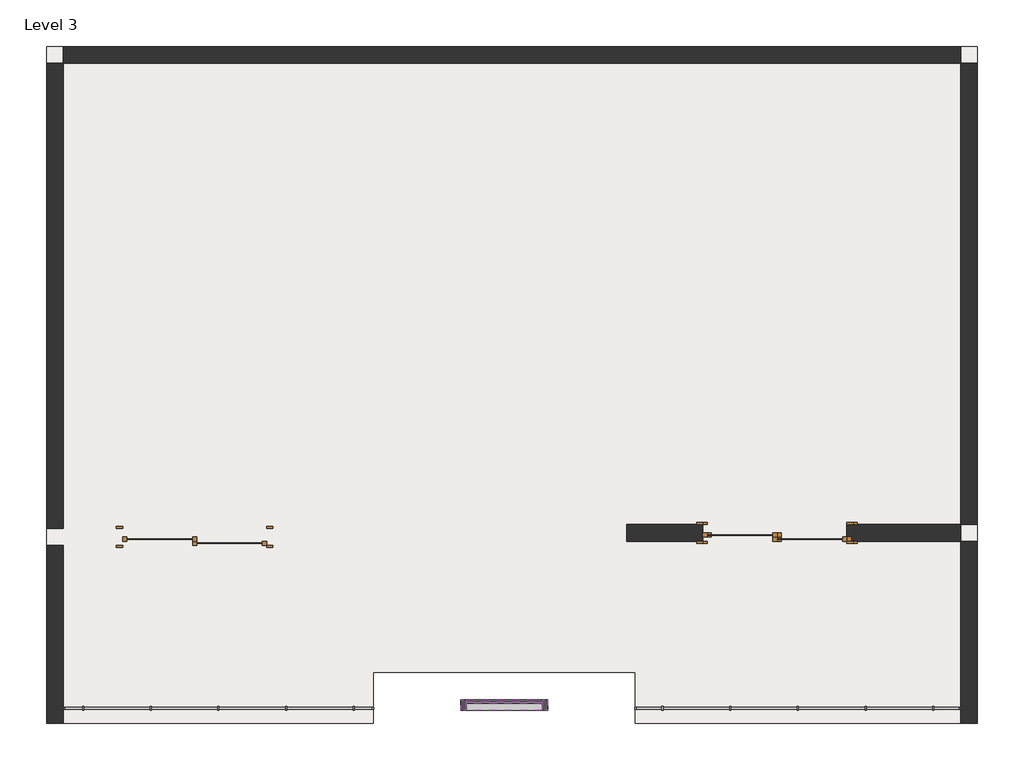
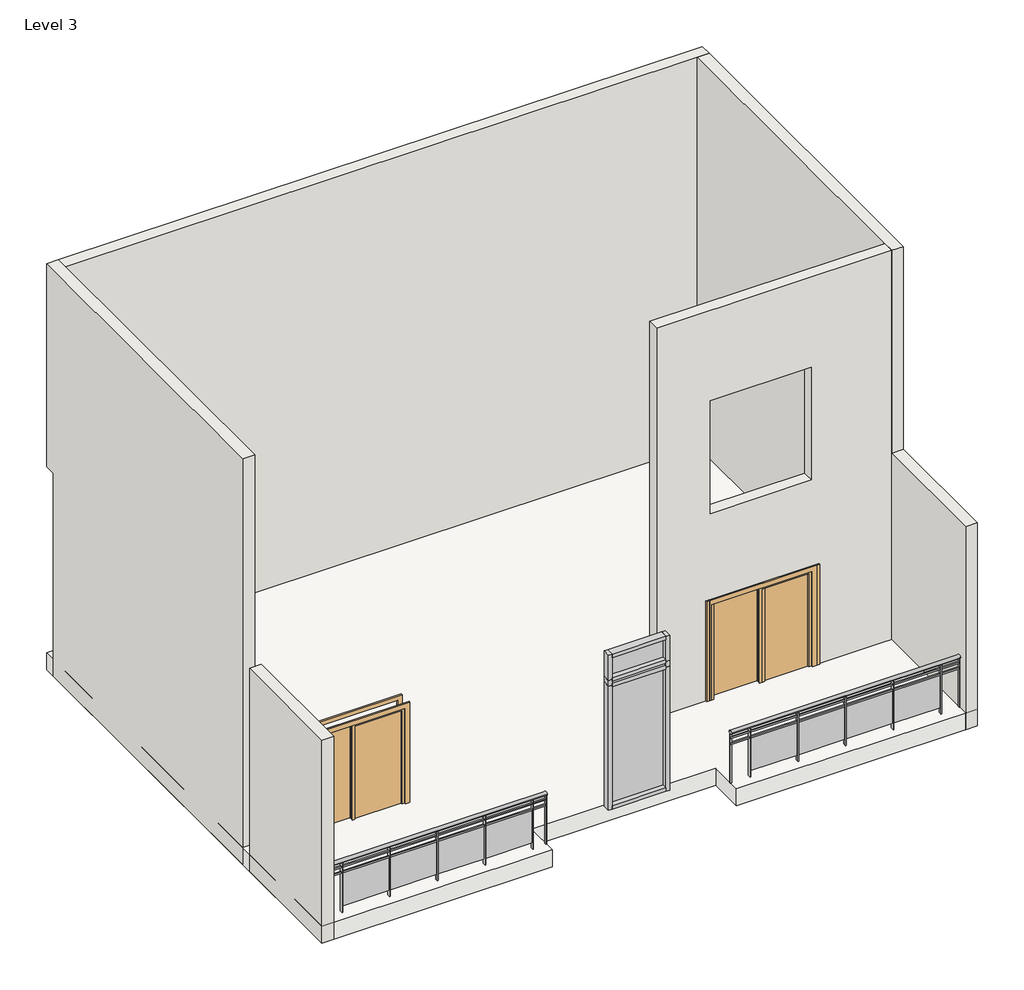
# One storey: 10 members, 6 walls, 3 doors, 3 plates, 2 railings, 1 roof.
"""IFC4 building model written with IfcOpenShell, lengths in millimetres."""

from ifc_helpers import new_model, si_unit, point, frame, origin, place, context, project, spatial, polyline, ellipse_curve, trimmed, outline, extrude, faceted_brep, transform, mapped, element, save
from ifc_brep_helpers import plane_surface, extruded_surface, advanced_brep
from components import door_076b30e0, member_d1708325, member_fb13da3b, member_15823cb3, member_73c23c35, member_410c6227, system_panel_glazed_14bb7e7b, system_panel_glazed_bdb1f896, system_panel_glazed_8073c085

model = new_model("IFC4")

# Units and contexts
model_context = context("Model", 3, world=origin())
ifc_project = project(units=[si_unit("LENGTHUNIT", "METRE", prefix="MILLI")], contexts=[model_context])

# Site, building, storey
site = spatial("IfcSite", under=ifc_project)
building = spatial("IfcBuilding", under=site)
storey = spatial("IfcBuildingStorey", under=building, Name="Level 3", Elevation=7315.2)

# Doors
placement = place(None, origin())
door_shape = door_076b30e0(model_context)
element("IfcDoor", 1, ObjectType="Door-Double-Sliding : 68\" x 80\"", at=placement, inside=storey, context=model_context, shape_type="MappedRepresentation", body=[
    mapped(door_shape, transform((-2271.8087885, 3717.6236997, 7315.2), x_axis=(-1.0, 0.0, 0.0), y_axis=(0.0, -1.0, 0.0), z_axis=(0.0, 0.0, 1.0))),
])
element("IfcDoor", 2, ObjectType="Door-Double-Sliding : 68\" x 80\"", at=placement, inside=storey, context=model_context, shape_type="MappedRepresentation", body=[
    mapped(door_shape, transform((-2221.0087885, 3717.6236997, 7315.2), x_axis=(-1.0, 0.0, 0.0), y_axis=(0.0, -1.0, 0.0), z_axis=(0.0, 0.0, 1.0))),
])
element("IfcDoor", 3, ObjectType="Door-Double-Sliding : 68\" x 80\"", at=placement, inside=storey, context=model_context, shape_type="MappedRepresentation", body=[
    mapped(door_shape, transform((-9238.1183714, 3666.8236997, 7315.2), x_axis=(-1.0, 0.0, 0.0), y_axis=(0.0, -1.0, 0.0), z_axis=(0.0, 0.0, 1.0))),
])

# Members
member_shape = member_d1708325(model_context)
element("IfcMember", 4, ObjectType="Rectangular Mullion : 2.5\" x 5\" rectangular", at=placement, inside=storey, context=model_context, shape_type="MappedRepresentation", body=[
    mapped(member_shape, transform((-6041.6537147, 1520.5236997, 10109.2), x_axis=(-1.0, 0.0, 0.0), y_axis=(0.0, -1.0, 0.0), z_axis=(0.0, 0.0, 1.0))),
])
member_2_shape = member_fb13da3b(model_context)
element("IfcMember", 5, ObjectType="Rectangular Mullion : 2.5\" x 5\" rectangular", at=placement, inside=storey, context=model_context, shape_type="MappedRepresentation", body=[
    mapped(member_2_shape, transform((-6041.6537147, 1520.5236997, 10210.8), x_axis=(-1.0, 0.0, 0.0), y_axis=(0.0, -1.0, 0.0), z_axis=(0.0, 0.0, 1.0))),
])
member_3_shape = member_15823cb3(model_context)
element("IfcMember", 6, ObjectType="Rectangular Mullion : 2.5\" x 5\" rectangular", at=placement, inside=storey, context=model_context, shape_type="MappedRepresentation", body=[
    mapped(member_3_shape, transform((-6041.6537147, 1520.5236997, 10668.0), x_axis=(-1.0, 0.0, 0.0), y_axis=(0.0, -1.0, 0.0), z_axis=(0.0, 0.0, 1.0))),
])
member_4_shape = member_73c23c35(model_context)
element("IfcMember", 7, ObjectType="Rectangular Mullion : 2.5\" x 5\" rectangular", at=placement, inside=storey, context=model_context, shape_type="MappedRepresentation", body=[
    mapped(member_4_shape, transform((-5978.1537147, 1520.5236997, 7874.0), x_axis=(0.0, 0.0, -1.0), y_axis=(0.0, -1.0, 0.0), z_axis=(-1.0, 0.0, 0.0))),
])
member_5_shape = member_410c6227(model_context)
element("IfcMember", 8, ObjectType="Rectangular Mullion : 2.5\" x 5\" rectangular", at=placement, inside=storey, context=model_context, shape_type="MappedRepresentation", body=[
    mapped(member_5_shape, transform((-5063.7537147, 1520.5236997, 10109.2), x_axis=(0.0, 0.0, 1.0), y_axis=(0.0, -1.0, 0.0), z_axis=(1.0, 0.0, 0.0))),
])
element("IfcMember", 9, ObjectType="Rectangular Mullion : 2.5\" x 5\" rectangular", at=placement, inside=storey, context=model_context, shape_type="MappedRepresentation", body=[
    mapped(member_5_shape, transform((-5063.7537147, 1520.5236997, 10210.8), x_axis=(0.0, 0.0, 1.0), y_axis=(0.0, -1.0, 0.0), z_axis=(1.0, 0.0, 0.0))),
])
element("IfcMember", 10, ObjectType="Rectangular Mullion : 2.5\" x 5\" rectangular", at=placement, inside=storey, context=model_context, shape_type="MappedRepresentation", body=[
    mapped(member_4_shape, transform((-5063.7537147, 1520.5236997, 10668.0), x_axis=(0.0, 0.0, 1.0), y_axis=(0.0, -1.0, 0.0), z_axis=(1.0, 0.0, 0.0))),
])
element("IfcMember", 11, ObjectType="Rectangular Mullion : 2.5\" x 5\" rectangular", at=placement, inside=storey, context=model_context, shape_type="MappedRepresentation", body=[
    mapped(member_2_shape, transform((-5000.2537147, 1520.5236997, 10109.2), x_axis=(1.0, 0.0, 0.0), y_axis=(0.0, -1.0, 0.0), z_axis=(0.0, 0.0, -1.0))),
])
element("IfcMember", 12, ObjectType="Rectangular Mullion : 2.5\" x 5\" rectangular", at=placement, inside=storey, context=model_context, shape_type="MappedRepresentation", body=[
    mapped(member_3_shape, transform((-5000.2537147, 1520.5236997, 10210.8), x_axis=(1.0, 0.0, 0.0), y_axis=(0.0, -1.0, 0.0), z_axis=(0.0, 0.0, -1.0))),
])
element("IfcMember", 13, ObjectType="Rectangular Mullion : 2.5\" x 5\" rectangular", at=placement, inside=storey, context=model_context, shape_type="MappedRepresentation", body=[
    mapped(member_shape, transform((-5000.2537147, 1520.5236997, 7874.0), x_axis=(1.0, 0.0, 0.0), y_axis=(0.0, -1.0, 0.0), z_axis=(0.0, 0.0, -1.0))),
])

# Plates
system_panel_glazed_shape = system_panel_glazed_14bb7e7b(model_context)
element("IfcPlate", 14, ObjectType="System Panel : Glazed", at=placement, inside=storey, context=model_context, shape_type="MappedRepresentation", body=[
    mapped(system_panel_glazed_shape, transform((-5520.9537147, 1520.5236997, 7937.5), x_axis=(1.0, 0.0, 0.0), y_axis=(0.0, 1.0, 0.0), z_axis=(0.0, 0.0, 1.0))),
])
system_panel_glazed_2_shape = system_panel_glazed_bdb1f896(model_context)
element("IfcPlate", 15, ObjectType="System Panel : Glazed", at=placement, inside=storey, context=model_context, shape_type="MappedRepresentation", body=[
    mapped(system_panel_glazed_2_shape, transform((-5520.9537147, 1520.5236997, 10242.55), x_axis=(1.0, 0.0, 0.0), y_axis=(0.0, 1.0, 0.0), z_axis=(0.0, 0.0, 1.0))),
])
system_panel_glazed_3_shape = system_panel_glazed_8073c085(model_context)
element("IfcPlate", 16, ObjectType="System Panel : Glazed", at=placement, inside=storey, context=model_context, shape_type="MappedRepresentation", body=[
    mapped(system_panel_glazed_3_shape, transform((-5520.9537147, 1520.5236997, 10140.95), x_axis=(1.0, 0.0, 0.0), y_axis=(0.0, 1.0, 0.0), z_axis=(0.0, 0.0, 1.0))),
])

# Railings
element("IfcRailing", 17, ObjectType="Glass Panel - Bottom Fill", at=placement, inside=storey, context=model_context, shape_type="SolidModel", body=[
    advanced_brep(
    [(-10812.9183714, 1520.5236997, 8534.4), (-10812.9183714, 1444.3236997, 8534.4), (-7091.896639, 1520.5236997, 8534.4), (-7091.896639, 1444.3236997, 8534.4)],
    [
        (0, 1, ellipse_curve(frame((-10812.9183714, 1482.4236997, 8534.4), z_axis=(-1.0, 0.0, 0.0), x_axis=(0.0, -1.0, 0.0)), 38.1, 28.575)),
        (1, 0, ellipse_curve(frame((-10812.9183714, 1482.4236997, 8534.4), z_axis=(-1.0, 0.0, 0.0), x_axis=(0.0, -1.0, 0.0)), 38.1, 28.575)),
        (2, 3, ellipse_curve(frame((-7091.896639, 1482.4236997, 8534.4), z_axis=(1.0, 0.0, 0.0), x_axis=(0.0, -1.0, 0.0)), 38.1, 28.575)),
        (3, 2, ellipse_curve(frame((-7091.896639, 1482.4236997, 8534.4), z_axis=(1.0, 0.0, 0.0), x_axis=(0.0, -1.0, 0.0)), 38.1, 28.575)),
        (0, 2),
        (3, 1),
    ],
    [
        plane_surface(frame((-10812.9183714, 1482.4236997, 8534.4), z_axis=(-1.0, 0.0, 0.0), x_axis=(0.0, 1.0, 0.0))),
        plane_surface(frame((-7091.896639, 1482.4236997, 8534.4), z_axis=(1.0, 0.0, 0.0), x_axis=(0.0, 1.0, 0.0))),
        extruded_surface(trimmed(ellipse_curve(frame((-7091.896639, 1482.4236997, 8534.4), z_axis=(-1.0, 0.0, 0.0), x_axis=(0.0, -1.0, 0.0)), 38.1, 28.575), [point((-7091.896639, 1520.5236997, 8534.4))], [point((-7091.896639, 1444.3236997, 8534.4))], True, "CARTESIAN"), (-3721.0217323999996, 0.0, 0.0), 3721.0217323999996),
        extruded_surface(trimmed(ellipse_curve(frame((-7091.896639, 1482.4236997, 8534.4), z_axis=(-1.0, 0.0, 0.0), x_axis=(0.0, -1.0, 0.0)), 38.1, 28.575), [point((-7091.896639, 1444.3236997, 8534.4))], [point((-7091.896639, 1520.5236997, 8534.4))], True, "CARTESIAN"), (-3721.0217323999996, 0.0, 0.0), 3721.0217323999996),
    ],
    [
        (0, [[1, 2]]),
        (1, [[3, 4]]),
        (2, [[-1, 5, -4, 6]]),
        (3, [[-2, -6, -3, -5]]),
    ],
),
    extrude(outline(polyline([(-10812.9183714, 1469.7236997), (-10812.9183714, 1495.1236997), (-7091.896639, 1495.1236997), (-7091.896639, 1469.7236997), (-10812.9183714, 1469.7236997)])), frame((0.0, 0.0, 8420.1), z_axis=(0.0, 0.0, 1.0), x_axis=(1.0, 0.0, 0.0)), (0.0, 0.0, 1.0), 25.4),
    extrude(outline(polyline([(-10812.9183714, 1469.7236997), (-10812.9183714, 1495.1236997), (-7091.896639, 1495.1236997), (-7091.896639, 1469.7236997), (-10812.9183714, 1469.7236997)])), frame((0.0, 0.0, 8318.5), z_axis=(0.0, 0.0, 1.0), x_axis=(1.0, 0.0, 0.0)), (0.0, 0.0, 1.0), 25.4),
    extrude(outline(polyline([(-7333.1575052, 1457.0236997), (-7333.1575052, 1507.8236997), (-7320.4575052, 1507.8236997), (-7320.4575052, 1457.0236997), (-7333.1575052, 1457.0236997)])), frame((0.0, 0.0, 7620.0), z_axis=(0.0, 0.0, 1.0), x_axis=(1.0, 0.0, 0.0)), (0.0, 0.0, 1.0), 885.6788223),
    extrude(outline(polyline([(-8139.6075052, 1488.9588567), (-7326.8075052, 1488.9588567), (-7326.8075052, 1482.6088567), (-8139.6075052, 1482.6088567), (-8139.6075052, 1488.9588567)])), frame((0.0, 0.0, 7721.6), z_axis=(0.0, 0.0, 1.0), x_axis=(1.0, 0.0, 0.0)), (0.0, 0.0, 1.0), 596.9),
    extrude(outline(polyline([(-8145.9575052, 1457.0236997), (-8145.9575052, 1507.8236997), (-8133.2575052, 1507.8236997), (-8133.2575052, 1457.0236997), (-8145.9575052, 1457.0236997)])), frame((0.0, 0.0, 7620.0), z_axis=(0.0, 0.0, 1.0), x_axis=(1.0, 0.0, 0.0)), (0.0, 0.0, 1.0), 885.6788223),
    extrude(outline(polyline([(-8952.4075052, 1488.9588567), (-8139.6075052, 1488.9588567), (-8139.6075052, 1482.6088567), (-8952.4075052, 1482.6088567), (-8952.4075052, 1488.9588567)])), frame((0.0, 0.0, 7721.6), z_axis=(0.0, 0.0, 1.0), x_axis=(1.0, 0.0, 0.0)), (0.0, 0.0, 1.0), 596.9),
    extrude(outline(polyline([(-8958.7575052, 1457.0236997), (-8958.7575052, 1507.8236997), (-8946.0575052, 1507.8236997), (-8946.0575052, 1457.0236997), (-8958.7575052, 1457.0236997)])), frame((0.0, 0.0, 7620.0), z_axis=(0.0, 0.0, 1.0), x_axis=(1.0, 0.0, 0.0)), (0.0, 0.0, 1.0), 885.6788223),
    extrude(outline(polyline([(-9765.2075052, 1488.9588567), (-8952.4075052, 1488.9588567), (-8952.4075052, 1482.6088567), (-9765.2075052, 1482.6088567), (-9765.2075052, 1488.9588567)])), frame((0.0, 0.0, 7721.6), z_axis=(0.0, 0.0, 1.0), x_axis=(1.0, 0.0, 0.0)), (0.0, 0.0, 1.0), 596.9),
    extrude(outline(polyline([(-9771.5575052, 1457.0236997), (-9771.5575052, 1507.8236997), (-9758.8575052, 1507.8236997), (-9758.8575052, 1457.0236997), (-9771.5575052, 1457.0236997)])), frame((0.0, 0.0, 7620.0), z_axis=(0.0, 0.0, 1.0), x_axis=(1.0, 0.0, 0.0)), (0.0, 0.0, 1.0), 885.6788223),
    extrude(outline(polyline([(-10578.0075052, 1488.9588567), (-9765.2075052, 1488.9588567), (-9765.2075052, 1482.6088567), (-10578.0075052, 1482.6088567), (-10578.0075052, 1488.9588567)])), frame((0.0, 0.0, 7721.6), z_axis=(0.0, 0.0, 1.0), x_axis=(1.0, 0.0, 0.0)), (0.0, 0.0, 1.0), 596.9),
    extrude(outline(polyline([(-10584.3575052, 1457.0236997), (-10584.3575052, 1507.8236997), (-10571.6575052, 1507.8236997), (-10571.6575052, 1457.0236997), (-10584.3575052, 1457.0236997)])), frame((0.0, 0.0, 7620.0), z_axis=(0.0, 0.0, 1.0), x_axis=(1.0, 0.0, 0.0)), (0.0, 0.0, 1.0), 885.6788223),
    extrude(outline(polyline([(-7104.596639, 1472.8986997), (-7104.596639, 1491.9486997), (-7085.546639, 1491.9486997), (-7085.546639, 1472.8986997), (-7104.596639, 1472.8986997)])), frame((0.0, 0.0, 7620.0), z_axis=(0.0, 0.0, 1.0), x_axis=(1.0, 0.0, 0.0)), (0.0, 0.0, 1.0), 885.6788223),
    extrude(outline(polyline([(-10819.2683714, 1472.8986997), (-10819.2683714, 1491.9486997), (-10800.2183714, 1491.9486997), (-10800.2183714, 1472.8986997), (-10819.2683714, 1472.8986997)])), frame((0.0, 0.0, 7620.0), z_axis=(0.0, 0.0, 1.0), x_axis=(1.0, 0.0, 0.0)), (0.0, 0.0, 1.0), 885.6788223),
])
element("IfcRailing", 18, ObjectType="Glass Panel - Bottom Fill", at=placement, inside=storey, context=model_context, shape_type="SolidModel", body=[
    advanced_brep(
    [(-3948.2087885, 1520.5236997, 8534.4), (-3948.2087885, 1444.3236997, 8534.4), (-43.3183714, 1520.5236997, 8534.4), (-43.3183714, 1444.3236997, 8534.4)],
    [
        (0, 1, ellipse_curve(frame((-3948.2087885, 1482.4236997, 8534.4), z_axis=(-1.0, 0.0, 0.0), x_axis=(0.0, -1.0, 0.0)), 38.1, 28.575)),
        (1, 0, ellipse_curve(frame((-3948.2087885, 1482.4236997, 8534.4), z_axis=(-1.0, 0.0, 0.0), x_axis=(0.0, -1.0, 0.0)), 38.1, 28.575)),
        (2, 3, ellipse_curve(frame((-43.3183714, 1482.4236997, 8534.4), z_axis=(1.0, 0.0, 0.0), x_axis=(0.0, -1.0, 0.0)), 38.1, 28.575)),
        (3, 2, ellipse_curve(frame((-43.3183714, 1482.4236997, 8534.4), z_axis=(1.0, 0.0, 0.0), x_axis=(0.0, -1.0, 0.0)), 38.1, 28.575)),
        (0, 2),
        (3, 1),
    ],
    [
        plane_surface(frame((-3948.2087885, 1482.4236997, 8534.4), z_axis=(-1.0, 0.0, 0.0), x_axis=(0.0, 1.0, 0.0))),
        plane_surface(frame((-43.3183714, 1482.4236997, 8534.4), z_axis=(1.0, 0.0, 0.0), x_axis=(0.0, 1.0, 0.0))),
        extruded_surface(trimmed(ellipse_curve(frame((-43.3183714, 1482.4236997, 8534.4), z_axis=(-1.0, 0.0, 0.0), x_axis=(0.0, -1.0, 0.0)), 38.1, 28.575), [point((-43.3183714, 1520.5236997, 8534.4))], [point((-43.3183714, 1444.3236997, 8534.4))], True, "CARTESIAN"), (-3904.8904171, 0.0, 0.0), 3904.8904171),
        extruded_surface(trimmed(ellipse_curve(frame((-43.3183714, 1482.4236997, 8534.4), z_axis=(-1.0, 0.0, 0.0), x_axis=(0.0, -1.0, 0.0)), 38.1, 28.575), [point((-43.3183714, 1444.3236997, 8534.4))], [point((-43.3183714, 1520.5236997, 8534.4))], True, "CARTESIAN"), (-3904.8904171, 0.0, 0.0), 3904.8904171),
    ],
    [
        (0, [[1, 2]]),
        (1, [[3, 4]]),
        (2, [[-1, 5, -4, 6]]),
        (3, [[-2, -6, -3, -5]]),
    ],
),
    extrude(outline(polyline([(-3948.2087885, 1469.7236997), (-3948.2087885, 1495.1236997), (-43.3183714, 1495.1236997), (-43.3183714, 1469.7236997), (-3948.2087885, 1469.7236997)])), frame((0.0, 0.0, 8420.1), z_axis=(0.0, 0.0, 1.0), x_axis=(1.0, 0.0, 0.0)), (0.0, 0.0, 1.0), 25.4),
    extrude(outline(polyline([(-3948.2087885, 1469.7236997), (-3948.2087885, 1495.1236997), (-43.3183714, 1495.1236997), (-43.3183714, 1469.7236997), (-3948.2087885, 1469.7236997)])), frame((0.0, 0.0, 8318.5), z_axis=(0.0, 0.0, 1.0), x_axis=(1.0, 0.0, 0.0)), (0.0, 0.0, 1.0), 25.4),
    extrude(outline(polyline([(-376.51358, 1457.0236997), (-376.51358, 1507.8236997), (-363.81358, 1507.8236997), (-363.81358, 1457.0236997), (-376.51358, 1457.0236997)])), frame((0.0, 0.0, 7620.0), z_axis=(0.0, 0.0, 1.0), x_axis=(1.0, 0.0, 0.0)), (0.0, 0.0, 1.0), 885.6788223),
    extrude(outline(polyline([(-1182.96358, 1488.9588567), (-370.16358, 1488.9588567), (-370.16358, 1482.6088567), (-1182.96358, 1482.6088567), (-1182.96358, 1488.9588567)])), frame((0.0, 0.0, 7721.6), z_axis=(0.0, 0.0, 1.0), x_axis=(1.0, 0.0, 0.0)), (0.0, 0.0, 1.0), 596.9),
    extrude(outline(polyline([(-1189.31358, 1457.0236997), (-1189.31358, 1507.8236997), (-1176.61358, 1507.8236997), (-1176.61358, 1457.0236997), (-1189.31358, 1457.0236997)])), frame((0.0, 0.0, 7620.0), z_axis=(0.0, 0.0, 1.0), x_axis=(1.0, 0.0, 0.0)), (0.0, 0.0, 1.0), 885.6788223),
    extrude(outline(polyline([(-1995.76358, 1488.9588567), (-1182.96358, 1488.9588567), (-1182.96358, 1482.6088567), (-1995.76358, 1482.6088567), (-1995.76358, 1488.9588567)])), frame((0.0, 0.0, 7721.6), z_axis=(0.0, 0.0, 1.0), x_axis=(1.0, 0.0, 0.0)), (0.0, 0.0, 1.0), 596.9),
    extrude(outline(polyline([(-2002.11358, 1457.0236997), (-2002.11358, 1507.8236997), (-1989.41358, 1507.8236997), (-1989.41358, 1457.0236997), (-2002.11358, 1457.0236997)])), frame((0.0, 0.0, 7620.0), z_axis=(0.0, 0.0, 1.0), x_axis=(1.0, 0.0, 0.0)), (0.0, 0.0, 1.0), 885.6788223),
    extrude(outline(polyline([(-2808.56358, 1488.9588567), (-1995.76358, 1488.9588567), (-1995.76358, 1482.6088567), (-2808.56358, 1482.6088567), (-2808.56358, 1488.9588567)])), frame((0.0, 0.0, 7721.6), z_axis=(0.0, 0.0, 1.0), x_axis=(1.0, 0.0, 0.0)), (0.0, 0.0, 1.0), 596.9),
    extrude(outline(polyline([(-2814.91358, 1457.0236997), (-2814.91358, 1507.8236997), (-2802.21358, 1507.8236997), (-2802.21358, 1457.0236997), (-2814.91358, 1457.0236997)])), frame((0.0, 0.0, 7620.0), z_axis=(0.0, 0.0, 1.0), x_axis=(1.0, 0.0, 0.0)), (0.0, 0.0, 1.0), 885.6788223),
    extrude(outline(polyline([(-3621.36358, 1488.9588567), (-2808.56358, 1488.9588567), (-2808.56358, 1482.6088567), (-3621.36358, 1482.6088567), (-3621.36358, 1488.9588567)])), frame((0.0, 0.0, 7721.6), z_axis=(0.0, 0.0, 1.0), x_axis=(1.0, 0.0, 0.0)), (0.0, 0.0, 1.0), 596.9),
    extrude(outline(polyline([(-3627.71358, 1457.0236997), (-3627.71358, 1507.8236997), (-3615.01358, 1507.8236997), (-3615.01358, 1457.0236997), (-3627.71358, 1457.0236997)])), frame((0.0, 0.0, 7620.0), z_axis=(0.0, 0.0, 1.0), x_axis=(1.0, 0.0, 0.0)), (0.0, 0.0, 1.0), 885.6788223),
    extrude(outline(polyline([(-56.0183714, 1472.8986997), (-56.0183714, 1491.9486997), (-36.9683714, 1491.9486997), (-36.9683714, 1472.8986997), (-56.0183714, 1472.8986997)])), frame((0.0, 0.0, 7620.0), z_axis=(0.0, 0.0, 1.0), x_axis=(1.0, 0.0, 0.0)), (0.0, 0.0, 1.0), 885.6788223),
    extrude(outline(polyline([(-3954.5587885, 1472.8986997), (-3954.5587885, 1491.9486997), (-3935.5087885, 1491.9486997), (-3935.5087885, 1472.8986997), (-3954.5587885, 1472.8986997)])), frame((0.0, 0.0, 7620.0), z_axis=(0.0, 0.0, 1.0), x_axis=(1.0, 0.0, 0.0)), (0.0, 0.0, 1.0), 885.6788223),
])

# Roof
element("IfcRoof", 19, ObjectType="Generic - 12\"", at=placement, inside=storey, context=model_context, shape_type="SweptSolid", body=[
    extrude(outline(polyline([(-11016.1183714, 9432.6236997), (159.8816286, 9432.6236997), (159.8816286, 1304.6236997), (-3948.2087885, 1304.6236997), (-3948.2087885, 1914.2236997), (-7091.896639, 1914.2236997), (-7091.896639, 1304.6236997), (-11016.1183714, 1304.6236997), (-11016.1183714, 9432.6236997)])), frame((0.0, 0.0, 7315.2), z_axis=(0.0, 0.0, 1.0), x_axis=(1.0, 0.0, 0.0)), (0.0, 0.0, 1.0), 304.8),
])

# Walls
element("IfcWall", 20, ObjectType="Generic - 8\"", at=placement, inside=storey, context=model_context, shape_type="Brep", body=[
    faceted_brep([(-10812.9183714, 3641.4236997, 14630.4), (-10812.9183714, 3641.4236997, 7315.2), (-10812.9183714, 9229.4236997, 7315.2), (-10812.9183714, 9229.4236997, 10972.8), (-10812.9183714, 9432.6236997, 10972.8), (-10812.9183714, 9432.6236997, 14630.4), (-10812.9183714, 9229.4236997, 14630.4), (-11016.1183714, 3641.4236997, 7315.2), (-11016.1183714, 3641.4236997, 14630.4), (-11016.1183714, 9432.6236997, 14630.4), (-11016.1183714, 9432.6236997, 10972.8), (-11016.1183714, 9229.4236997, 10972.8), (-11016.1183714, 9229.4236997, 7315.2)], [[[0, 1, 2, 3, 4, 5, 6]], [[7, 8, 9, 10, 11, 12]], [[2, 1, 7, 12]], [[0, 6, 5, 9, 8]], [[0, 8, 7, 1]], [[10, 4, 3, 11]], [[3, 2, 12, 11]], [[5, 4, 10, 9]]]),
])
element("IfcWall", 21, ObjectType="Generic - 8\"", at=placement, inside=storey, context=model_context, shape_type="Brep", body=[
    faceted_brep([(-10812.9183714, 9229.4236997, 14630.4), (-10812.9183714, 9229.4236997, 7315.2), (-43.3183714, 9229.4236997, 7315.2), (-43.3183714, 9229.4236997, 10972.8), (159.8816286, 9229.4236997, 10972.8), (159.8816286, 9229.4236997, 14630.4), (-43.3183714, 9229.4236997, 14630.4), (-10812.9183714, 9432.6236997, 7315.2), (-10812.9183714, 9432.6236997, 10972.8), (-10812.9183714, 9432.6236997, 14630.4), (159.8816286, 9432.6236997, 14630.4), (159.8816286, 9432.6236997, 10972.8), (-43.3183714, 9432.6236997, 10972.8), (-43.3183714, 9432.6236997, 7315.2)], [[[0, 1, 2, 3, 4, 5, 6]], [[7, 8, 9, 10, 11, 12, 13]], [[2, 1, 7, 13]], [[0, 6, 5, 10, 9]], [[0, 9, 8, 7, 1]], [[11, 4, 3, 12]], [[3, 2, 13, 12]], [[5, 4, 11, 10]]]),
])
element("IfcWall", 22, ObjectType="Generic - 8\"", at=placement, inside=storey, context=model_context, shape_type="Brep", body=[
    faceted_brep([(-43.3183714, 9229.4236997, 14630.4), (-43.3183714, 9229.4236997, 7315.2), (-43.3183714, 3692.2236997, 7315.2), (-43.3183714, 3692.2236997, 10972.8), (-43.3183714, 3489.0236997, 10972.8), (-43.3183714, 3489.0236997, 14630.4), (-43.3183714, 3692.2236997, 14630.4), (159.8816286, 9229.4236997, 7315.2), (159.8816286, 9229.4236997, 10972.8), (159.8816286, 9229.4236997, 14630.4), (159.8816286, 3489.0236997, 14630.4), (159.8816286, 3489.0236997, 10972.8), (159.8816286, 3692.2236997, 10972.8), (159.8816286, 3692.2236997, 7315.2)], [[[0, 1, 2, 3, 4, 5, 6]], [[7, 8, 9, 10, 11, 12, 13]], [[2, 1, 7, 13]], [[0, 6, 5, 10, 9]], [[0, 9, 8, 7, 1]], [[11, 4, 3, 12]], [[3, 2, 13, 12]], [[5, 4, 11, 10]]]),
])
element("IfcWall", 23, ObjectType="Generic - 8\"", at=placement, inside=storey, context=model_context, shape_type="Brep", body=[
    faceted_brep([(-3135.4087885, 3692.2236997, 9347.2), (-3135.4087885, 3692.2236997, 7315.2), (-4049.8087885, 3692.2236997, 7315.2), (-4049.8087885, 3692.2236997, 14630.4), (-43.3183714, 3692.2236997, 14630.4), (-43.3183714, 3692.2236997, 7315.2), (-1357.4087885, 3692.2236997, 7315.2), (-1408.2087885, 3692.2236997, 7315.2), (-1408.2087885, 3692.2236997, 9347.2), (-1408.2087885, 3692.2236997, 13004.8), (-3135.4087885, 3692.2236997, 13004.8), (-3135.4087885, 3692.2236997, 10972.8), (-1408.2087885, 3692.2236997, 10972.8), (-4049.8087885, 3489.0236997, 7315.2), (-3135.4087885, 3489.0236997, 7315.2), (-3135.4087885, 3489.0236997, 9347.2), (-1408.2087885, 3489.0236997, 9347.2), (-1408.2087885, 3489.0236997, 7315.2), (-1357.4087885, 3489.0236997, 7315.2), (-43.3183714, 3489.0236997, 7315.2), (-43.3183714, 3489.0236997, 10972.8), (-43.3183714, 3489.0236997, 14630.4), (-4049.8087885, 3489.0236997, 14630.4), (-1408.2087885, 3489.0236997, 13004.8), (-1408.2087885, 3489.0236997, 10972.8), (-3135.4087885, 3489.0236997, 10972.8), (-3135.4087885, 3489.0236997, 13004.8)], [[[0, 1, 2, 3, 4, 5, 6, 7, 8], [9, 10, 11, 12]], [[13, 14, 15, 16, 17, 18, 19, 20, 21, 22], [23, 24, 25, 26]], [[2, 1, 14, 13]], [[7, 6, 5, 19, 18, 17]], [[3, 2, 13, 22]], [[4, 3, 22, 21]], [[4, 21, 20, 19, 5]], [[17, 16, 8, 7]], [[15, 14, 1, 0]], [[16, 15, 0, 8]], [[24, 23, 9, 12]], [[25, 24, 12, 11]], [[26, 25, 11, 10]], [[23, 26, 10, 9]]]),
])
element("IfcWall", 24, ObjectType="Generic - 8\"", at=placement, inside=storey, context=model_context, shape_type="SweptSolid", body=[
    extrude(outline(polyline([(-11016.1183714, 1304.6236997), (-11016.1183714, 3438.2236997), (-10812.9183714, 3438.2236997), (-10812.9183714, 1304.6236997), (-11016.1183714, 1304.6236997)])), frame((0.0, 0.0, 7315.2), z_axis=(0.0, 0.0, 1.0), x_axis=(1.0, 0.0, 0.0)), (0.0, 0.0, 1.0), 3657.6),
])
element("IfcWall", 25, ObjectType="Generic - 8\"", at=placement, inside=storey, context=model_context, shape_type="SweptSolid", body=[
    extrude(outline(polyline([(-43.3183714, 1304.6236997), (-43.3183714, 3489.0236997), (159.8816286, 3489.0236997), (159.8816286, 1304.6236997), (-43.3183714, 1304.6236997)])), frame((0.0, 0.0, 7315.2), z_axis=(0.0, 0.0, 1.0), x_axis=(1.0, 0.0, 0.0)), (0.0, 0.0, 1.0), 3657.6),
])

save(model, "model.ifc")

# Revit data of these elements
# Type "Door-Double-Sliding : 68\" x 80\""
#   Type Mark = "11"
#   Construction Type Id = "opn-d45"
#   Assembly Code = "C1020"
#   Analytic Construction = "Wood frame, double glass door "
#   Thickness = 0' - 2"
#   Thermal Resistance (R) = 1.8150 (h·ft²·°F)/BTU
#   Heat Transfer Coefficient (U) = 0.5510 BTU/(h·ft²·°F)
#   Height = 6' - 8"
#   Rail Width = 0' - 2"
#   Stiles = 0' - 2"
#   Trim Projection Ext = 0' - 1"
#   Trim Projection Int = 0' - 1"
#   Trim Width = 0' - 3"
#   Width = 5' - 8"
#   Define Thermal Properties by = 1
#   Glazing = Glass
#   Panel Material = Wood - Birch - Solid Stained Light Low Gloss
#   Trim Material = Paint - Sienna
#   Visual Light Transmittance = 0
#   Solar Heat Gain Coefficient = 0
#   Function = (empty or 0)
#   Wall Closure = (empty or 0)
# Type "Rectangular Mullion : 2.5\" x 5\" rectangular"
#   built-in parameter 1007304 = 0.416667 (stored number, unit not read)
#   built-in parameter 1007301 = 0.104167 (stored number, unit not read)
#   built-in parameter 1007300 = 0.104167 (stored number, unit not read)
# Type "System Panel : Glazed"
#   Construction Type Id = "GSP4R"
#   Analytic Construction = "1/8 in Pilkington single glazing"
#   Visual Light Transmittance = 0.9
#   Solar Heat Gain Coefficient = 0.86
#   Heat Transfer Coefficient (U) = 1.18115 BTU/(h·ft²·°F)
# Type "Glass Panel - Bottom Fill"
#   Assembly Code = "C2010400"
#   built-in parameter 1008612 = 0.0416667 (stored number, unit not read)
#   built-in parameter 1008611 = 0.0416667 (stored number, unit not read)
#   built-in parameter 1008609 = 0.333333 (stored number, unit not read)
#   built-in parameter 1008604 = 0.166667 (stored number, unit not read)
#   built-in parameter 1008603 = 0.166667 (stored number, unit not read)
#   Railing Height = 3' - 0"
#   built-in parameter 1008630 = 2
#   built-in parameter 1008610 = 2
#   built-in parameter 1008618 = Baluster - Square : 3/4"
# Type "Generic - 12\""
#   Assembly Code = "B1020"
#   Layers, outside or top first: 1' - 0" no material (function 1)
# Type "Generic - 8\""
#   Assembly Code = "B2010"
#   Layers, outside or top first: 0' - 8" no material (function 1)
# Elements 1, 2, 3 (IfcDoor, "Door-Double-Sliding : 68\" x 80\"")
#   Phase Created = New Construction
#   Materials on its faces: "Paint - Sienna", "Wood - Birch - Solid Stained Light Low Gloss", "Glass"
# Elements 4, 5, 6, 7, 8, 9, 10, 11, 12, 13 (IfcMember, "Rectangular Mullion : 2.5\" x 5\" rectangular")
#   Phase Created = New Construction
#   Materials on its faces: "Aluminum"
# Elements 14, 15, 16 (IfcPlate, "System Panel : Glazed")
#   Phase Created = New Construction
#   Materials on its faces: "Glass"
# Elements 17, 18 (IfcRailing, "Glass Panel - Bottom Fill")
#   built-in parameter 1008621 = 1 (stored number, unit not read)
#   Phase Created = New Construction
#   Materials on its faces: "Glass"
# Element 19 (IfcRoof, "Generic - 12\"")
#   built-in parameter 1001705 = 25 (stored number, unit not read)
#   built-in parameter 1001710 = 33615
#   Phase Created = New Construction
#   Materials on its faces: "Default Roof"
# Elements 20, 21, 22, 23 (IfcWall, "Generic - 8\"")
#   Top Offset = 0' - 0"
#   Base Offset = 0' - 0"
#   Unconnected Height = 24' - 0"
#   wall height = 24' - 0"
#   Phase Created = New Construction
#   Base Constraint = Level 3
#   Materials on its faces: "Default Wall"
# Elements 24, 25 (IfcWall, "Generic - 8\"")
#   Top Offset = 0' - 0"
#   Base Offset = 0' - 0"
#   Unconnected Height = 12' - 0"
#   wall height = 12' - 0"
#   Phase Created = New Construction
#   Base Constraint = Level 3
#   Materials on its faces: "Default Wall"
# Materials
#   "Glass": class "Glass", colour RGB 0 128 192, transparency 0.75, Description = "Soda Lime Glass", Cost = 0
#   "Wood - Birch - Solid Stained Light Low Gloss": class "Wood", colour RGB 210 159 95, transparency 0, Cost = 0
#   "Paint - Sienna": colour RGB 118 70 51, transparency 0, Cost = 0
#   "Aluminum": class "Metal", colour RGB 247 247 247, transparency 0, Description = "Aluminum 6061", Cost = 0
#   "Default Roof": colour RGB 88 101 114, transparency 0
#   "Default Wall": colour RGB 128 128 128, transparency 0
